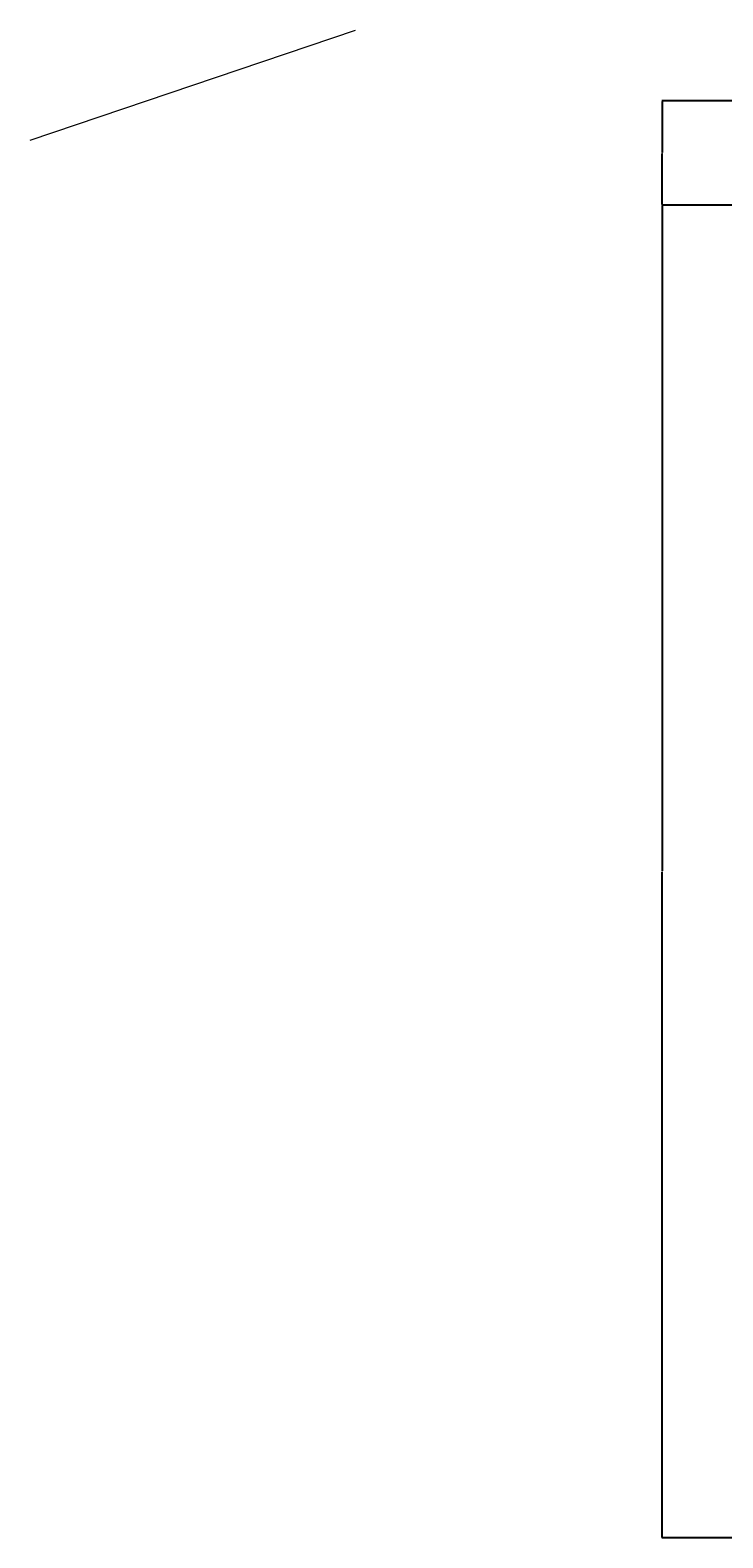
# Model space of a CAD drawing. Units: inches. Extents: x -1085 to 1941, y 1514 to 2348.
# Tile 1 of 9: x -1085 to -836, y 1725 to 2268. Entities that reach past the tile are written whole.
import ezdxf

# ---------------------------------------------------------------- set-up
doc = ezdxf.new("R2010")
doc.units = ezdxf.units.IN
doc.layers.add('A-ANNO-DIMS', color=2, linetype='Continuous', lineweight=18)
doc.layers.add('A-DETL-REFR', color=8, linetype='Continuous', lineweight=13)
doc.styles.get("Standard").update_dxf_attribs({"font": 'arial.ttf'})
doc.dimstyles.get("Standard").update_dxf_attribs({"dimtxt": 0.18, "dimasz": 0.18, "dimexe": 0.18, "dimexo": 0.0625, "dimgap": 0.09, "dimtad": 0, "dimtih": 1, "dimtoh": 1, "dimdec": 4, "dimzin": 0, "dimdsep": 46, "dimtxsty": 'Standard', "dimcen": 0.09, "dimadec": 0, "dimazin": 0, "dimtfac": 1, "dimtdec": 4, "dimtofl": 0, "dimtmove": 0, "dimatfit": 3, "dimfxl": 1, "dimtolj": 1, "dimtzin": 0, "dimarcsym": 0})

# ---------------------------------------------------------------- blocks, each defined once
blk = doc.blocks.new('*D97')
at = {"layer": 'A-ANNO-DIMS', "color": 0, "lineweight": -2, "transparency": 16777216}
for p, q in [((-791.17, 2205.38), (-857.78, 2205.38)), ((-857.6, 2205.2), (-857.6, 1965.57)), ((-857.6, 1725.56), (-857.6, 1965.2)), ((-791.17, 1725.38), (-857.78, 1725.38))]:
    blk.add_line(p, q, dxfattribs=at)
at = {"layer": 'A-ANNO-DIMS', "color": 0, "transparency": 16777216}
for points in [[(-857.63, 2205.2), (-857.57, 2205.2), (-857.6, 2205.38)], [(-857.63, 1725.56), (-857.57, 1725.56), (-857.6, 1725.38)]]:
    blk.add_solid(points, dxfattribs=at)
at = {"layer": 'Defpoints', "color": 0, "transparency": 16777216}
for p in [(-791.1, 2205.38), (-857.6, 1725.38), (-791.1, 1725.38)]:
    blk.add_point(p, dxfattribs=at)
at = {"layer": 'A-ANNO-DIMS', "color": 0, "transparency": 16777216, "insert": (-857.6, 1965.38), "char_height": 0.18, "attachment_point": 5}
blk.add_mtext('\\A1;480', dxfattribs=at)
blk = doc.blocks.new('*D99')
at = {"layer": 'A-ANNO-DIMS', "color": 0, "lineweight": -2, "transparency": 16777216}
for p, q in [((-828.67, 2242.88), (-857.78, 2242.88)), ((-857.6, 2242.7), (-857.6, 2224.32)), ((-857.6, 2205.56), (-857.6, 2223.95)), ((-791.17, 2205.38), (-857.78, 2205.38))]:
    blk.add_line(p, q, dxfattribs=at)
at = {"layer": 'A-ANNO-DIMS', "color": 0, "transparency": 16777216}
for points in [[(-857.63, 2242.7), (-857.57, 2242.7), (-857.6, 2242.88)], [(-857.63, 2205.56), (-857.57, 2205.56), (-857.6, 2205.38)]]:
    blk.add_solid(points, dxfattribs=at)
at = {"layer": 'Defpoints', "color": 0, "transparency": 16777216}
for p in [(-828.6, 2242.88), (-857.6, 2205.38), (-791.1, 2205.38)]:
    blk.add_point(p, dxfattribs=at)
at = {"layer": 'A-ANNO-DIMS', "color": 0, "transparency": 16777216, "insert": (-857.6, 2224.13), "char_height": 0.18, "attachment_point": 5}
blk.add_mtext('\\A1;37.5', dxfattribs=at)

msp = doc.modelspace()

# ---------------------------------------------------------------- linework, layer by layer
at = {"layer": 'A-DETL-REFR'}
msp.add_line((-1085.1892, 2228.75), (-968.0534, 2268.3905), dxfattribs=at)

# ---------------------------------------------------------------- dimensions: what is measured, and where the dimension line sits
at = {"layer": 'A-ANNO-DIMS'}
for base, p1, p2, override, picture, middle in [((-857.6032, 2205.3835), (-828.6032, 2242.8835), (-791.1032, 2205.3835), {"dimdec": 1, "dimlfac": 1, "dimrnd": 0, "dimzin": 0, "dimdsep": 46, "dimlunit": 2}, '*D99', (-857.6032, 2224.1335)), ((-857.6032, 1725.3835), (-791.1032, 2205.3835), (-791.1032, 1725.3835), {"dimdec": 0, "dimlfac": 1, "dimrnd": 0, "dimzin": 0, "dimdsep": 46, "dimlunit": 2}, '*D97', (-857.6032, 1965.3835))]:
    dim = msp.add_linear_dim(base=base, p1=p1, p2=p2, angle=90, dimstyle='Standard', override=override, dxfattribs=at)
    dim.commit()
    dim.dimension.update_dxf_attribs({"geometry": picture, "text_midpoint": middle})

doc.saveas('drawing.dxf')
